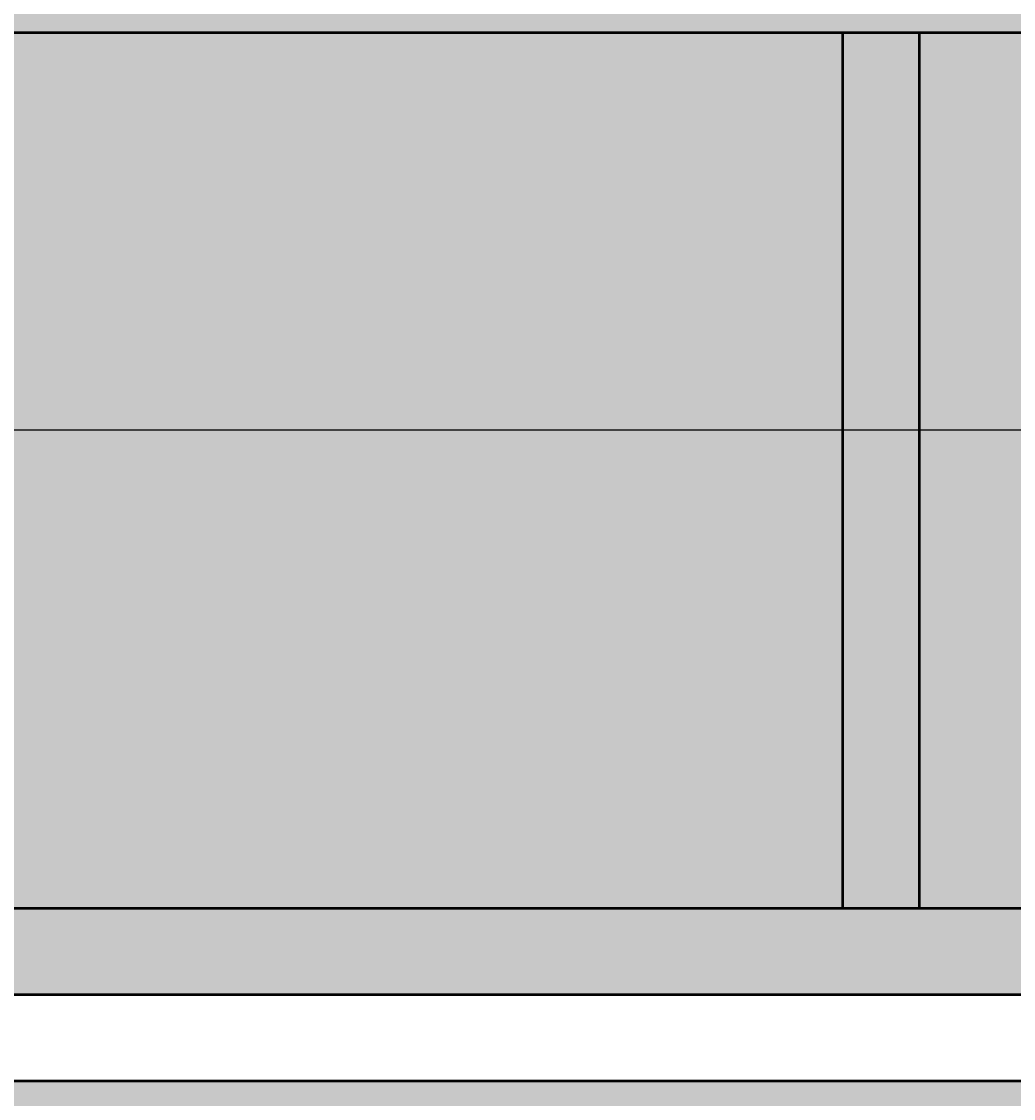
# Model space of a CAD drawing. Units: inches. Extents: x -12 to 334, y -10 to 186.
# Tile 42 of 77: x 152 to 175, y 65 to 90. Entities that reach past the tile are written whole.
import ezdxf

# ---------------------------------------------------------------- set-up
doc = ezdxf.new("R2010")
doc.units = ezdxf.units.IN
doc.header["$MEASUREMENT"] = 0
for name, color, linetype, lineweight in [('M-DIMS', 2, 'Continuous', 18), ('M-EQPM', 7, 'Continuous', 50), ('M-EQPM-PATT', 8, 'Continuous', 18)]:
    doc.layers.add(name, color=color, linetype=linetype, lineweight=lineweight)
doc.styles.get("Standard").update_dxf_attribs({"font": 'arial.ttf'})
doc.dimstyles.get("Standard").update_dxf_attribs({"dimtxt": 0.18, "dimasz": 0.18, "dimexe": 0.18, "dimexo": 0.0625, "dimgap": 0.09, "dimtad": 0, "dimtih": 1, "dimtoh": 1, "dimdec": 4, "dimzin": 0, "dimdsep": 46, "dimtxsty": 'Standard', "dimcen": 0.09, "dimadec": 0, "dimazin": 0, "dimtfac": 1, "dimtdec": 4, "dimtofl": 0, "dimtmove": 0, "dimatfit": 3, "dimfxl": 1, "dimtolj": 1, "dimtzin": 0, "dimarcsym": 0})

# ---------------------------------------------------------------- blocks, each defined once
blk = doc.blocks.new('*D1')
at = {"layer": 'Defpoints', "color": 0, "transparency": 16777216}
for p in [(281.426, 91.899), (3.376, 80.692), (281.426, 14.304)]:
    blk.add_point(p, dxfattribs=at)
at = {"layer": 'M-DIMS', "color": 0, "lineweight": -2, "transparency": 16777216}
for p, q in [((281.426, 91.836), (281.426, 14.124)), ((3.376, 80.629), (3.376, 14.124)), ((3.556, 14.304), (141.935, 14.304)), ((281.246, 14.304), (142.867, 14.304))]:
    blk.add_line(p, q, dxfattribs=at)
at = {"layer": 'M-DIMS', "color": 0, "transparency": 16777216}
for points in [[(3.556, 14.334), (3.556, 14.274), (3.376, 14.304)], [(281.246, 14.334), (281.246, 14.274), (281.426, 14.304)]]:
    blk.add_solid(points, dxfattribs=at)
at = {"layer": 'M-DIMS', "color": 0, "transparency": 16777216, "insert": (142.401, 14.304), "char_height": 0.18, "attachment_point": 5}
blk.add_mtext('\\A1;278.05', dxfattribs=at)
blk = doc.blocks.new('*D17')
at = {"layer": 'Defpoints', "color": 0, "transparency": 16777216}
for p in [(106.177, 102.896), (105.892, 56.321), (295.976, 56.321)]:
    blk.add_point(p, dxfattribs=at)
at = {"layer": 'M-DIMS', "color": 0, "lineweight": -2, "transparency": 16777216}
for p, q in [((106.24, 102.896), (296.156, 102.896)), ((295.976, 102.716), (295.976, 79.79)), ((295.976, 56.501), (295.976, 79.426)), ((105.954, 56.321), (296.156, 56.321))]:
    blk.add_line(p, q, dxfattribs=at)
at = {"layer": 'M-DIMS', "color": 0, "transparency": 16777216}
for points in [[(295.946, 102.716), (296.006, 102.716), (295.976, 102.896)], [(295.946, 56.501), (296.006, 56.501), (295.976, 56.321)]]:
    blk.add_solid(points, dxfattribs=at)
at = {"layer": 'M-DIMS', "color": 0, "transparency": 16777216, "insert": (295.976, 79.608), "char_height": 0.18, "attachment_point": 5}
blk.add_mtext('\\A1;46.575', dxfattribs=at)
blk = doc.blocks.new('*D35')
at = {"layer": 'Defpoints', "color": 0, "transparency": 16777216}
for p in [(216.428, 98.108), (-11.174, 61.105), (216.428, 61.105)]:
    blk.add_point(p, dxfattribs=at)
at = {"layer": 'M-DIMS', "color": 0, "lineweight": -2, "transparency": 16777216}
for p, q in [((216.365, 98.108), (-11.354, 98.108)), ((-11.174, 97.928), (-11.174, 79.788)), ((-11.174, 61.285), (-11.174, 79.424)), ((216.365, 61.105), (-11.354, 61.105))]:
    blk.add_line(p, q, dxfattribs=at)
at = {"layer": 'M-DIMS', "color": 0, "transparency": 16777216}
for points in [[(-11.204, 97.928), (-11.144, 97.928), (-11.174, 98.108)], [(-11.204, 61.285), (-11.144, 61.285), (-11.174, 61.105)]]:
    blk.add_solid(points, dxfattribs=at)
at = {"layer": 'M-DIMS', "color": 0, "transparency": 16777216, "insert": (-11.174, 79.606), "char_height": 0.18, "attachment_point": 5}
blk.add_mtext('\\A1;37', dxfattribs=at)
blk = doc.blocks.new('*D39')
at = {"layer": 'Defpoints', "color": 0, "transparency": 16777216}
for p in [(279.726, 80.692), (-11.174, 45.854), (269.381, 45.854)]:
    blk.add_point(p, dxfattribs=at)
at = {"layer": 'M-DIMS', "color": 0, "lineweight": -2, "transparency": 16777216}
for p, q in [((279.664, 80.692), (-11.354, 80.692)), ((-11.174, 80.512), (-11.174, 63.455)), ((-11.174, 46.034), (-11.174, 63.091)), ((269.318, 45.854), (-11.354, 45.854))]:
    blk.add_line(p, q, dxfattribs=at)
at = {"layer": 'M-DIMS', "color": 0, "transparency": 16777216}
for points in [[(-11.204, 80.512), (-11.144, 80.512), (-11.174, 80.692)], [(-11.204, 46.034), (-11.144, 46.034), (-11.174, 45.854)]]:
    blk.add_solid(points, dxfattribs=at)
at = {"layer": 'M-DIMS', "color": 0, "transparency": 16777216, "insert": (-11.174, 63.273), "char_height": 0.18, "attachment_point": 5}
blk.add_mtext('\\A1;34.84', dxfattribs=at)

msp = doc.modelspace()

# ---------------------------------------------------------------- hatches: boundary and pattern name
at = {"layer": 'M-EQPM-PATT'}
h = msp.add_hatch(color=256, dxfattribs=at)
h.set_gradient(color1=(205, 32, 39), color2=(205, 32, 39), tint=1)
h.paths.add_polyline_path([(64.5, 80.754), (64.5, 89.8963), (226.6083, 89.8963, -1), (226.6083, 69.6117), (64.5, 69.6117), (64.5, 78.754), (4.4744, 78.754, 0.384914), (23.5807, 61.4872), (37.1002, 61.4872), (37.1002, 33.6752), (53.1002, 33.6752), (53.1002, 61.4872), (64.5, 61.4872), (64.5, 63.6117), (226.6083, 63.6117, 1), (226.6083, 95.8963), (64.5, 95.8963), (64.5, 99.8958), (53.1002, 99.8958), (53.1002, 127.7078), (37.1002, 127.7078), (37.1002, 99.8958), (23.5807, 99.8958, 0.4132606), (4.3766, 80.754)])
h.paths.add_polyline_path([(64.5, 91.8963), (64.5, 93.8963), (226.6083, 93.8963, -1), (226.6083, 65.6117), (64.5, 65.6117), (64.5, 67.6117), (226.6083, 67.6117, 1), (226.6083, 91.8963)], flags=16)
h = msp.add_hatch(color=256, dxfattribs=at)
h.set_gradient(color1=(99, 100, 102), color2=(99, 100, 102), tint=1)
h.paths.add_polyline_path([(72.9244, 95.8963), (75.9244, 95.8963), (75.9244, 109.0583), (72.9244, 109.0583)])
h.paths.add_polyline_path([(72.9244, 50.4497), (75.9244, 50.4497), (75.9244, 63.6117), (72.9244, 63.6117)])
h.paths.add_polyline_path([(75.9244, 91.8963), (75.9244, 93.8963), (72.9244, 93.8963), (72.9244, 91.8963)])
h.paths.add_polyline_path([(75.9244, 65.6117), (75.9244, 67.6117), (72.9244, 67.6117), (72.9244, 65.6117)])
h.paths.add_polyline_path([(129.093, 69.6117), (130.8573, 69.6117), (130.8573, 89.8963), (129.093, 89.8963)])
h.paths.add_polyline_path([(129.093, 98.1081), (129.093, 95.8963), (130.8573, 95.8963), (130.8573, 98.1081)])
h.paths.add_polyline_path([(130.8573, 61.1045), (130.8573, 63.6117), (129.093, 63.6117), (129.093, 61.1045)])
h.paths.add_polyline_path([(170.9079, 69.6117), (172.6722, 69.6117), (172.6722, 89.8963), (170.9079, 89.8963)])
h.paths.add_polyline_path([(172.6722, 95.8963), (172.6722, 98.1081), (170.9079, 98.1081), (170.9079, 95.8963)])
h.paths.add_polyline_path([(170.9079, 61.1045), (172.6722, 61.1045), (172.6722, 63.6117), (170.9079, 63.6117)])
h.paths.add_polyline_path([(218.1922, 63.6117), (216.4278, 63.6117), (216.4278, 61.1045), (218.1922, 61.1045)])
h.paths.add_polyline_path([(216.4278, 69.6117), (218.1922, 69.6117), (218.1922, 89.8963), (216.4278, 89.8963)])
h.paths.add_polyline_path([(216.4278, 95.8963), (218.1922, 95.8963), (218.1922, 98.1081), (216.4278, 98.1081)])
h = msp.add_hatch(color=256, dxfattribs=at)
h.set_gradient(color1=(94, 103, 175), color2=(94, 103, 175), tint=1)
h.paths.add_polyline_path([(129.093, 89.8963), (86.8879, 89.8963), (86.8879, 69.6117), (129.093, 69.6117)], flags=17)
h.paths.add_polyline_path([(170.9079, 89.8963), (130.8573, 89.8963), (130.8573, 69.6117), (170.9079, 69.6117)], flags=17)
h.paths.add_polyline_path([(216.4278, 89.8963), (172.6722, 89.8963), (172.6722, 69.6117), (216.4278, 69.6117)], flags=17)
h.paths.add_polyline_path([(245.9354, 82.6969), (247.9354, 82.6969), (247.9354, 46.8541), (268.3808, 46.8541, 0.0998398), (279.7263, 80.6915), (251.9801, 80.6915, 0.4142136), (231.7758, 100.8958), (84.7229, 100.8958), (84.7229, 109.0583), (83.7229, 109.0583), (83.7229, 95.8963), (129.093, 95.8963), (129.093, 98.1081), (130.8573, 98.1081), (130.8573, 95.8963), (170.9079, 95.8963), (170.9079, 98.1081), (172.6722, 98.1081), (172.6722, 95.8963), (216.4278, 95.8963), (216.4278, 98.1081), (218.1922, 98.1081), (218.1922, 95.8963), (226.6083, 95.8963, -1), (226.6083, 63.6117), (218.1922, 63.6117), (218.1922, 61.1045), (216.4278, 61.1045), (216.4278, 63.6117), (172.6722, 63.6117), (172.6722, 61.1045), (170.9079, 61.1045), (170.9079, 63.6117), (130.8573, 63.6117), (130.8573, 61.1045), (129.093, 61.1045), (129.093, 63.6117), (87.8879, 63.6117), (87.8879, 56.3205), (105.8919, 56.3205), (105.8919, 28.8541), (115.8919, 28.8541), (115.8919, 46.8541), (222.5761, 46.8541), (222.5761, 30.8541), (232.5761, 30.8541), (232.5761, 46.8541), (245.9354, 46.8541)])
h.paths.add_polyline_path([(86.8879, 89.8963), (75.9244, 89.8963), (75.9244, 69.6117), (86.8879, 69.6117)])
h.paths.add_polyline_path([(83.7229, 109.0583), (75.9244, 109.0583), (75.9244, 95.8963), (83.7229, 95.8963)])
h.paths.add_polyline_path([(226.6083, 89.8963), (218.1922, 89.8963), (218.1922, 69.6117), (226.6083, 69.6117, 1)], flags=17)

# ---------------------------------------------------------------- linework, layer by layer
at = {"layer": 'M-EQPM'}
for points in [[(64.5, 65.6117), (226.6083, 65.6117, 1), (226.6083, 93.8963), (64.5, 93.8963)], [(64.5, 67.6117), (226.6083, 67.6117, 1), (226.6083, 91.8963), (64.5, 91.8963)], [(64.5, 69.6117), (226.6083, 69.6117, 1), (226.6083, 89.8963), (64.5, 89.8963)]]:
    msp.add_lwpolyline(points, format="xyb", dxfattribs=at)
for points in [[(170.9079, 69.6117), (170.9079, 89.8963)], [(172.6722, 89.8963), (172.6722, 69.6117)]]:
    msp.add_lwpolyline(points, dxfattribs=at)

# ---------------------------------------------------------------- dimensions: what is measured, and where the dimension line sits
at = {"layer": 'M-DIMS'}
for base, p1, p2, override, picture, middle in [((295.9756, 56.3205), (106.1771, 102.8958), (105.8919, 56.3205), {"dimdec": 3, "dimlfac": 1, "dimrnd": 0, "dimzin": 0, "dimdsep": 46, "dimlunit": 2}, '*D17', (295.9756, 79.6082)), ((-11.1736, 61.1045), (216.4278, 98.1081), (216.4278, 61.1045), {"dimdec": 0, "dimlfac": 1, "dimrnd": 0, "dimzin": 0, "dimdsep": 46, "dimlunit": 2}, '*D35', (-11.1735, 79.6063)), ((-11.1736, 45.8541), (279.7263, 80.6915), (269.3808, 45.8541), {"dimdec": 2, "dimlfac": 1, "dimrnd": 0, "dimzin": 0, "dimdsep": 46, "dimlunit": 2}, '*D39', (-11.1735, 63.2728))]:
    dim = msp.add_linear_dim(base=base, p1=p1, p2=p2, angle=90, dimstyle='Standard', override=override, dxfattribs=at)
    dim.commit()
    dim.dimension.update_dxf_attribs({"geometry": picture, "text_midpoint": middle})
dim = msp.add_linear_dim(base=(281.4256, 14.3041), p1=(3.3765, 80.6915), p2=(281.4256, 91.8988), dimstyle='Standard', override={"dimdec": 2, "dimlfac": 1, "dimrnd": 0, "dimzin": 0, "dimdsep": 46, "dimlunit": 2}, dxfattribs=at)
dim.commit()
dim.dimension.update_dxf_attribs({"geometry": '*D1', "text_midpoint": (142.401, 14.3041)})

doc.saveas('drawing.dxf')
